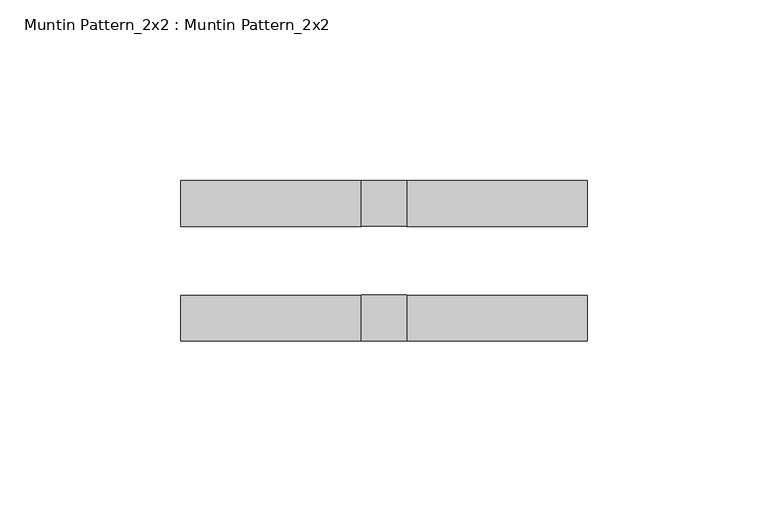
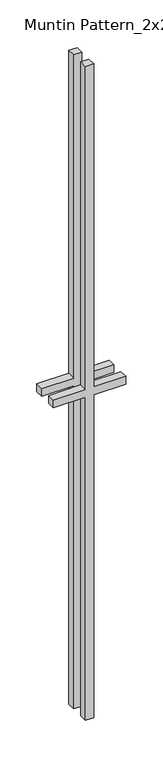
"""IFC4 building model written with IfcOpenShell, lengths in millimetres: proxy geometry, Muntin Pattern_2x2 : Muntin Pattern_2x2."""

from ifc_helpers import new_model, si_unit, frame, origin, place, context, project, spatial, polyline, outline, extrude, source, transform, mapped, element, save


def muntin_pattern_2x2_muntin_pattern_2x2_a9af9031(model_context):
    return source(origin(), model_context, "Body", "SweptSolid", [
        extrude(outline(polyline([(546.1, -6.35), (546.1, -56.3378825), (533.4, -56.3378825), (533.4, -6.35), (0.0, -6.35), (0.0, 6.35), (533.4, 6.35), (533.4, 56.3378825), (546.1, 56.3378825), (546.1, 6.35), (1079.5, 6.35), (1079.5, -6.35), (546.1, -6.35)])), frame((0.0, -22.225, 0.0), z_axis=(0.0, 1.0, 0.0), x_axis=(0.0, 0.0, 1.0)), (0.0, 0.0, 1.0), 12.7),
        extrude(outline(polyline([(546.1, -6.35), (546.1, -56.3378825), (533.4, -56.3378825), (533.4, -6.35), (0.0, -6.35), (0.0, 6.35), (533.4, 6.35), (533.4, 56.3378825), (546.1, 56.3378825), (546.1, 6.35), (1079.5, 6.35), (1079.5, -6.35), (546.1, -6.35)])), frame((0.0, 9.525, 0.0), z_axis=(0.0, 1.0, 0.0), x_axis=(0.0, 0.0, 1.0)), (0.0, 0.0, 1.0), 12.7),
    ])


if __name__ == "__main__":
    model = new_model("IFC4")
    model_context = context("Model", 3, world=origin())
    ifc_project = project(units=[si_unit("LENGTHUNIT", "METRE", prefix="MILLI")], contexts=[model_context])
    site = spatial("IfcSite", under=ifc_project)
    building = spatial("IfcBuilding", under=site)
    placement = place(None, origin())
    muntin_pattern_2x2_muntin_pattern_2x2_shape = muntin_pattern_2x2_muntin_pattern_2x2_a9af9031(model_context)
    element("IfcBuildingElementProxy", 1, Name="Muntin Pattern_2x2 : Muntin Pattern_2x2", ObjectType="Muntin Pattern_2x2 : Muntin Pattern_2x2", at=placement, inside=building, context=model_context, shape_type="MappedRepresentation", body=[
        mapped(muntin_pattern_2x2_muntin_pattern_2x2_shape, transform((0.0, 0.0, 0.0), x_axis=(1.0, 0.0, 0.0), y_axis=(0.0, 1.0, 0.0), z_axis=(0.0, 0.0, 1.0))),
    ])
    save(model, "model.ifc")

# Revit data of these elements
# Type "Muntin Pattern_2x2 : Muntin Pattern_2x2"
#   Width [instance default] = 4' - 0"
#   Thickness = 0' - 0 1/2"
#   Height [instance default] = 4' - 0"
#   Distance = 0' - 0 3/4"
#   Interior Material [instance default] = none
#   Exterior Material [instance default] = none
#   Default Elevation = 0
# Element 1 (IfcBuildingElementProxy, "Muntin Pattern_2x2 : Muntin Pattern_2x2")
#   Width = 0' - 4.43605"
#   Height = 3' - 6 1/2"
#   Interior Material = Wood - Stained
#   Exterior Material = Clad - White
#   Materials on its faces: "Clad - White", "Wood - Stained"
# Materials
#   "Clad - White": class "Wood", colour RGB 242 242 238, transparency 0, Cost = 0
#   "Wood - Stained": class "Wood", colour RGB 224 178 126, transparency 0, Cost = 0
